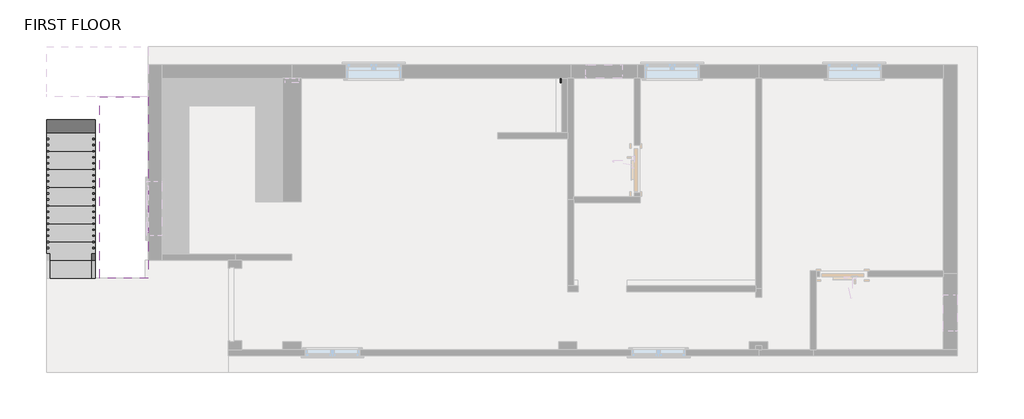
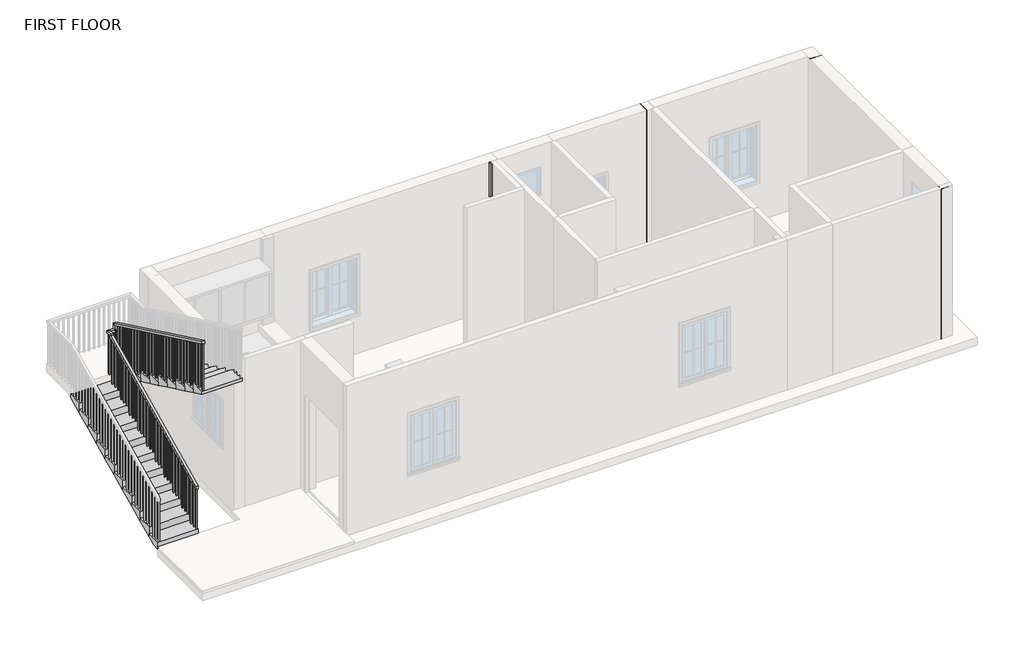
# One storey, part 2 of 3: 4 columns, 2 stair flights, 1 railing.
"""IFC4 building model written with IfcOpenShell, lengths in millimetres."""

from ifc_helpers import new_model, si_unit, frame, origin, place, context, project, spatial, polyline, outline, extrude, faceted_brep, element, save

model = new_model("IFC4")

# Units and contexts
model_context = context("Model", 3, world=origin())
ifc_project = project(units=[si_unit("LENGTHUNIT", "METRE", prefix="MILLI")], contexts=[model_context])

# Site, building, storey
site = spatial("IfcSite", under=ifc_project)
building = spatial("IfcBuilding", under=site)
storey = spatial("IfcBuildingStorey", under=building, Name="FIRST FLOOR", Elevation=3200.4)

# Columns
placement = place(None, origin())
element("IfcColumn", 1, ObjectType="Rectangular Column : 9\" X 12\"", at=placement, inside=storey, context=model_context, shape_type="Brep", body=[
    faceted_brep([(8641.6408773, 5102.5642852, 3200.4), (8870.2408773, 5102.5642852, 3200.4), (8870.2408773, 4797.7642852, 3200.4), (8641.6408773, 4797.7642852, 3200.4), (8641.6408773, 4873.9642852, 3200.4), (8641.6408773, 5102.5642852, 6400.8), (8870.2408773, 5102.5642852, 6400.8), (8870.2408773, 4797.7642852, 6400.8), (8641.6408773, 4797.7642852, 6400.8), (8641.6408773, 4873.9642852, 6400.8)], [[[0, 1, 2, 3, 4]], [[5, 6, 1, 0]], [[6, 7, 2, 1]], [[7, 8, 3, 2]], [[8, 9, 5, 0, 4, 3]], [[5, 9, 8, 7, 6]]]),
])
element("IfcColumn", 2, ObjectType="Rectangular Column : 9\" X 12\"", at=placement, inside=storey, context=model_context, shape_type="Brep", body=[
    faceted_brep([(5390.4408773, 4873.9642852, 3200.4), (5390.4408773, 5102.5642852, 3200.4), (5542.8408773, 5102.5642852, 3200.4), (5542.8408773, 4873.9642852, 3200.4), (5492.0408773, 4873.9642852, 3200.4), (5390.4408773, 4873.9642852, 6400.8), (5390.4408773, 5102.5642852, 6400.8), (5542.8408773, 5102.5642852, 6400.8), (5542.8408773, 4873.9642852, 6400.8), (5492.0408773, 4873.9642852, 6400.8)], [[[0, 1, 2, 3, 4]], [[1, 0, 5, 6]], [[1, 6, 7, 2]], [[5, 0, 4, 3, 8, 9]], [[6, 5, 9, 8, 7]], [[3, 2, 7, 8]]]),
])
element("IfcColumn", 3, ObjectType="Rectangular Column : 9\" X 12\"", at=placement, inside=storey, context=model_context, shape_type="SweptSolid", body=[
    extrude(outline(polyline([(2240.8408773, 4797.7642852), (2215.4408773, 4797.7642852), (2215.4408773, 4873.9642852), (2240.8408773, 4873.9642852), (2240.8408773, 4797.7642852)])), frame((0.0, 0.0, 3200.4), z_axis=(0.0, 0.0, 1.0), x_axis=(1.0, 0.0, 0.0)), (0.0, 0.0, 1.0), 3200.4),
])
element("IfcColumn", 4, ObjectType="Rectangular Column : 9\" X 12\"", at=placement, inside=storey, context=model_context, shape_type="SweptSolid", body=[
    extrude(outline(polyline([(8870.2408773, 225.7642852), (8641.6408773, 225.7642852), (8641.6408773, 327.3642852), (8870.2408773, 327.3642852), (8870.2408773, 225.7642852)])), frame((0.0, 0.0, 3200.4), z_axis=(0.0, 0.0, 1.0), x_axis=(1.0, 0.0, 0.0)), (0.0, 0.0, 1.0), 3200.4),
])

# Railing
element("IfcRailing", 5, ObjectType="Handrail - Rectangular", at=placement, inside=storey, context=model_context, shape_type="SolidModel", body=[
    faceted_brep([(-5633.1591227, 1521.1642852, 4260.2727273), (-5633.1591227, 1521.1642852, 4203.9834559), (-5582.3591227, 1521.1642852, 4203.9834559), (-5582.3591227, 1521.1642852, 4260.2727273), (-5633.1591227, 4492.9642852, 5678.6318182), (-5633.1591227, 4543.7642852, 5646.5880014), (-5582.3591227, 4543.7642852, 5646.5880014), (-5582.3591227, 4492.9642852, 5678.6318182), (-5633.1591227, 4492.9642852, 5715.0), (-5633.1591227, 4543.7642852, 5664.2), (-5582.3591227, 4543.7642852, 5664.2), (-5582.3591227, 4492.9642852, 5715.0), (-5633.1591227, 4619.9642852, 5715.0), (-5633.1591227, 4619.9642852, 5664.2), (-5582.3591227, 4569.1642852, 5664.2), (-5582.3591227, 4569.1642852, 5715.0), (-5506.1591227, 4619.9642852, 5715.0), (-5506.1591227, 4619.9642852, 5664.2), (-5506.1591227, 4569.1642852, 5664.2), (-5506.1591227, 4569.1642852, 5715.0), (-5480.7591227, 4619.9642852, 5715.0), (-5480.7591227, 4569.1642852, 5715.0), (-5480.7591227, 4569.1642852, 5664.2), (-5480.7591227, 4619.9642852, 5664.2)], [[[0, 1, 2, 3]], [[1, 0, 4, 5]], [[2, 1, 5, 6]], [[3, 2, 6, 7]], [[0, 3, 7, 4]], [[5, 4, 8, 9]], [[6, 5, 9, 10]], [[7, 6, 10, 11]], [[4, 7, 11, 8]], [[9, 8, 12, 13]], [[10, 9, 13, 14]], [[11, 10, 14, 15]], [[8, 11, 15, 12]], [[13, 12, 16, 17]], [[14, 13, 17, 18]], [[15, 14, 18, 19]], [[12, 15, 19, 16]], [[20, 21, 22, 23]], [[17, 16, 20, 23]], [[18, 17, 23, 22]], [[19, 18, 22, 21]], [[16, 19, 21, 20]]]),
    faceted_brep([(-5506.1591227, 4619.9642852, 5715.0), (-5455.3591227, 4619.9642852, 5664.2), (-5455.3591227, 4569.1642852, 5664.2), (-5506.1591227, 4569.1642852, 5715.0), (-5506.1591227, 4619.9642852, 5836.2272727), (-5506.1591227, 4569.1642852, 5804.1834559), (-5455.3591227, 4569.1642852, 5804.1834559), (-5455.3591227, 4619.9642852, 5836.2272727)], [[[0, 1, 2, 3]], [[4, 5, 6, 7]], [[1, 0, 4, 7]], [[2, 1, 7, 6]], [[3, 2, 6, 5]], [[0, 3, 5, 4]]]),
    faceted_brep([(-5455.3591227, 4619.9642852, 5836.2272727), (-5455.3591227, 4569.1642852, 5804.1834559), (-5506.1591227, 4569.1642852, 5804.1834559), (-5506.1591227, 4619.9642852, 5836.2272727), (-5455.3591227, 1521.1642852, 7315.2), (-5506.1591227, 1521.1642852, 7315.2), (-5506.1591227, 1521.1642852, 7258.9107287), (-5455.3591227, 1521.1642852, 7258.9107287)], [[[0, 1, 2, 3]], [[4, 5, 6, 7]], [[1, 0, 4, 7]], [[2, 1, 7, 6]], [[3, 2, 6, 5]], [[0, 3, 5, 4]]]),
    extrude(outline(polyline([(1537.0392852, 7251.3340241), (1556.0892852, 7242.2419787), (1556.0892852, 6255.3272727), (1537.0392852, 6255.3272727), (1537.0392852, 7251.3340241)])), frame((-5490.2841227, 0.0, 0.0), z_axis=(1.0, 0.0, 0.0), x_axis=(0.0, 1.0, 0.0)), (0.0, 0.0, 1.0), 19.05),
    extrude(outline(polyline([(1638.6392852, 7202.843115), (1657.6892852, 7193.7510696), (1657.6892852, 6255.3272727), (1638.6392852, 6255.3272727), (1638.6392852, 7202.843115)])), frame((-5490.2841227, 0.0, 0.0), z_axis=(1.0, 0.0, 0.0), x_axis=(0.0, 1.0, 0.0)), (0.0, 0.0, 1.0), 19.05),
    extrude(outline(polyline([(1740.2392852, 7154.3522059), (1759.2892852, 7145.2601605), (1759.2892852, 6255.3272727), (1740.2392852, 6255.3272727), (1740.2392852, 7154.3522059)])), frame((-5490.2841227, 0.0, 0.0), z_axis=(1.0, 0.0, 0.0), x_axis=(0.0, 1.0, 0.0)), (0.0, 0.0, 1.0), 19.05),
    extrude(outline(polyline([(1841.8392852, 7105.8612969), (1860.8892852, 7096.7692514), (1860.8892852, 6109.8545455), (1841.8392852, 6109.8545455), (1841.8392852, 7105.8612969)])), frame((-5490.2841227, 0.0, 0.0), z_axis=(1.0, 0.0, 0.0), x_axis=(0.0, 1.0, 0.0)), (0.0, 0.0, 1.0), 19.05),
    extrude(outline(polyline([(1943.4392852, 7057.3703878), (1962.4892852, 7048.2783423), (1962.4892852, 6109.8545455), (1943.4392852, 6109.8545455), (1943.4392852, 7057.3703878)])), frame((-5490.2841227, 0.0, 0.0), z_axis=(1.0, 0.0, 0.0), x_axis=(0.0, 1.0, 0.0)), (0.0, 0.0, 1.0), 19.05),
    extrude(outline(polyline([(2045.0392852, 7008.8794787), (2064.0892852, 6999.7874332), (2064.0892852, 6109.8545455), (2045.0392852, 6109.8545455), (2045.0392852, 7008.8794787)])), frame((-5490.2841227, 0.0, 0.0), z_axis=(1.0, 0.0, 0.0), x_axis=(0.0, 1.0, 0.0)), (0.0, 0.0, 1.0), 19.05),
    extrude(outline(polyline([(2146.6392852, 6960.3885696), (2165.6892852, 6951.2965241), (2165.6892852, 5964.3818182), (2146.6392852, 5964.3818182), (2146.6392852, 6960.3885696)])), frame((-5490.2841227, 0.0, 0.0), z_axis=(1.0, 0.0, 0.0), x_axis=(0.0, 1.0, 0.0)), (0.0, 0.0, 1.0), 19.05),
    extrude(outline(polyline([(2248.2392852, 6911.8976605), (2267.2892852, 6902.805615), (2267.2892852, 5964.3818182), (2248.2392852, 5964.3818182), (2248.2392852, 6911.8976605)])), frame((-5490.2841227, 0.0, 0.0), z_axis=(1.0, 0.0, 0.0), x_axis=(0.0, 1.0, 0.0)), (0.0, 0.0, 1.0), 19.05),
    extrude(outline(polyline([(2349.8392852, 6863.4067514), (2368.8892852, 6854.3147059), (2368.8892852, 5964.3818182), (2349.8392852, 5964.3818182), (2349.8392852, 6863.4067514)])), frame((-5490.2841227, 0.0, 0.0), z_axis=(1.0, 0.0, 0.0), x_axis=(0.0, 1.0, 0.0)), (0.0, 0.0, 1.0), 19.05),
    extrude(outline(polyline([(2451.4392852, 6814.9158423), (2470.4892852, 6805.8237969), (2470.4892852, 5818.9090909), (2451.4392852, 5818.9090909), (2451.4392852, 6814.9158423)])), frame((-5490.2841227, 0.0, 0.0), z_axis=(1.0, 0.0, 0.0), x_axis=(0.0, 1.0, 0.0)), (0.0, 0.0, 1.0), 19.05),
    extrude(outline(polyline([(2553.0392852, 6766.4249332), (2572.0892852, 6757.3328878), (2572.0892852, 5818.9090909), (2553.0392852, 5818.9090909), (2553.0392852, 6766.4249332)])), frame((-5490.2841227, 0.0, 0.0), z_axis=(1.0, 0.0, 0.0), x_axis=(0.0, 1.0, 0.0)), (0.0, 0.0, 1.0), 19.05),
    extrude(outline(polyline([(2654.6392852, 6717.9340241), (2673.6892852, 6708.8419787), (2673.6892852, 5818.9090909), (2654.6392852, 5818.9090909), (2654.6392852, 6717.9340241)])), frame((-5490.2841227, 0.0, 0.0), z_axis=(1.0, 0.0, 0.0), x_axis=(0.0, 1.0, 0.0)), (0.0, 0.0, 1.0), 19.05),
    extrude(outline(polyline([(2756.2392852, 6669.443115), (2775.2892852, 6660.3510696), (2775.2892852, 5673.4363636), (2756.2392852, 5673.4363636), (2756.2392852, 6669.443115)])), frame((-5490.2841227, 0.0, 0.0), z_axis=(1.0, 0.0, 0.0), x_axis=(0.0, 1.0, 0.0)), (0.0, 0.0, 1.0), 19.05),
    extrude(outline(polyline([(2857.8392852, 6620.9522059), (2876.8892852, 6611.8601605), (2876.8892852, 5673.4363636), (2857.8392852, 5673.4363636), (2857.8392852, 6620.9522059)])), frame((-5490.2841227, 0.0, 0.0), z_axis=(1.0, 0.0, 0.0), x_axis=(0.0, 1.0, 0.0)), (0.0, 0.0, 1.0), 19.05),
    extrude(outline(polyline([(2959.4392852, 6572.4612969), (2978.4892852, 6563.3692514), (2978.4892852, 5673.4363636), (2959.4392852, 5673.4363636), (2959.4392852, 6572.4612969)])), frame((-5490.2841227, 0.0, 0.0), z_axis=(1.0, 0.0, 0.0), x_axis=(0.0, 1.0, 0.0)), (0.0, 0.0, 1.0), 19.05),
    extrude(outline(polyline([(3061.0392852, 6523.9703878), (3080.0892852, 6514.8783423), (3080.0892852, 5527.9636364), (3061.0392852, 5527.9636364), (3061.0392852, 6523.9703878)])), frame((-5490.2841227, 0.0, 0.0), z_axis=(1.0, 0.0, 0.0), x_axis=(0.0, 1.0, 0.0)), (0.0, 0.0, 1.0), 19.05),
    extrude(outline(polyline([(3162.6392852, 6475.4794787), (3181.6892852, 6466.3874332), (3181.6892852, 5527.9636364), (3162.6392852, 5527.9636364), (3162.6392852, 6475.4794787)])), frame((-5490.2841227, 0.0, 0.0), z_axis=(1.0, 0.0, 0.0), x_axis=(0.0, 1.0, 0.0)), (0.0, 0.0, 1.0), 19.05),
    extrude(outline(polyline([(3264.2392852, 6426.9885696), (3283.2892852, 6417.8965241), (3283.2892852, 5527.9636364), (3264.2392852, 5527.9636364), (3264.2392852, 6426.9885696)])), frame((-5490.2841227, 0.0, 0.0), z_axis=(1.0, 0.0, 0.0), x_axis=(0.0, 1.0, 0.0)), (0.0, 0.0, 1.0), 19.05),
    extrude(outline(polyline([(3365.8392852, 6378.4976605), (3384.8892852, 6369.405615), (3384.8892852, 5382.4909091), (3365.8392852, 5382.4909091), (3365.8392852, 6378.4976605)])), frame((-5490.2841227, 0.0, 0.0), z_axis=(1.0, 0.0, 0.0), x_axis=(0.0, 1.0, 0.0)), (0.0, 0.0, 1.0), 19.05),
    extrude(outline(polyline([(3467.4392852, 6330.0067514), (3486.4892852, 6320.9147059), (3486.4892852, 5382.4909091), (3467.4392852, 5382.4909091), (3467.4392852, 6330.0067514)])), frame((-5490.2841227, 0.0, 0.0), z_axis=(1.0, 0.0, 0.0), x_axis=(0.0, 1.0, 0.0)), (0.0, 0.0, 1.0), 19.05),
    extrude(outline(polyline([(3569.0392852, 6281.5158423), (3588.0892852, 6272.4237969), (3588.0892852, 5382.4909091), (3569.0392852, 5382.4909091), (3569.0392852, 6281.5158423)])), frame((-5490.2841227, 0.0, 0.0), z_axis=(1.0, 0.0, 0.0), x_axis=(0.0, 1.0, 0.0)), (0.0, 0.0, 1.0), 19.05),
    extrude(outline(polyline([(3670.6392852, 6233.0249332), (3689.6892852, 6223.9328878), (3689.6892852, 5237.0181818), (3670.6392852, 5237.0181818), (3670.6392852, 6233.0249332)])), frame((-5490.2841227, 0.0, 0.0), z_axis=(1.0, 0.0, 0.0), x_axis=(0.0, 1.0, 0.0)), (0.0, 0.0, 1.0), 19.05),
    extrude(outline(polyline([(3772.2392852, 6184.5340241), (3791.2892852, 6175.4419787), (3791.2892852, 5237.0181818), (3772.2392852, 5237.0181818), (3772.2392852, 6184.5340241)])), frame((-5490.2841227, 0.0, 0.0), z_axis=(1.0, 0.0, 0.0), x_axis=(0.0, 1.0, 0.0)), (0.0, 0.0, 1.0), 19.05),
    extrude(outline(polyline([(3873.8392852, 6136.043115), (3892.8892852, 6126.9510696), (3892.8892852, 5237.0181818), (3873.8392852, 5237.0181818), (3873.8392852, 6136.043115)])), frame((-5490.2841227, 0.0, 0.0), z_axis=(1.0, 0.0, 0.0), x_axis=(0.0, 1.0, 0.0)), (0.0, 0.0, 1.0), 19.05),
    extrude(outline(polyline([(3975.4392852, 6087.5522059), (3994.4892852, 6078.4601605), (3994.4892852, 5091.5454545), (3975.4392852, 5091.5454545), (3975.4392852, 6087.5522059)])), frame((-5490.2841227, 0.0, 0.0), z_axis=(1.0, 0.0, 0.0), x_axis=(0.0, 1.0, 0.0)), (0.0, 0.0, 1.0), 19.05),
    extrude(outline(polyline([(4077.0392852, 6039.0612969), (4096.0892852, 6029.9692514), (4096.0892852, 5091.5454545), (4077.0392852, 5091.5454545), (4077.0392852, 6039.0612969)])), frame((-5490.2841227, 0.0, 0.0), z_axis=(1.0, 0.0, 0.0), x_axis=(0.0, 1.0, 0.0)), (0.0, 0.0, 1.0), 19.05),
    extrude(outline(polyline([(4178.6392852, 5990.5703878), (4197.6892852, 5981.4783423), (4197.6892852, 5091.5454545), (4178.6392852, 5091.5454545), (4178.6392852, 5990.5703878)])), frame((-5490.2841227, 0.0, 0.0), z_axis=(1.0, 0.0, 0.0), x_axis=(0.0, 1.0, 0.0)), (0.0, 0.0, 1.0), 19.05),
    extrude(outline(polyline([(4280.2392852, 5942.0794787), (4299.2892852, 5932.9874332), (4299.2892852, 4946.0727273), (4280.2392852, 4946.0727273), (4280.2392852, 5942.0794787)])), frame((-5490.2841227, 0.0, 0.0), z_axis=(1.0, 0.0, 0.0), x_axis=(0.0, 1.0, 0.0)), (0.0, 0.0, 1.0), 19.05),
    extrude(outline(polyline([(4381.8392852, 5893.5885696), (4400.8892852, 5884.4965241), (4400.8892852, 4946.0727273), (4381.8392852, 4946.0727273), (4381.8392852, 5893.5885696)])), frame((-5490.2841227, 0.0, 0.0), z_axis=(1.0, 0.0, 0.0), x_axis=(0.0, 1.0, 0.0)), (0.0, 0.0, 1.0), 19.05),
    extrude(outline(polyline([(4483.4392852, 5845.0976605), (4502.4892852, 5836.005615), (4502.4892852, 4946.0727273), (4483.4392852, 4946.0727273), (4483.4392852, 5845.0976605)])), frame((-5490.2841227, 0.0, 0.0), z_axis=(1.0, 0.0, 0.0), x_axis=(0.0, 1.0, 0.0)), (0.0, 0.0, 1.0), 19.05),
    extrude(outline(polyline([(-5515.6841227, 4585.0392852), (-5515.6841227, 4604.0892852), (-5496.6341227, 4604.0892852), (-5496.6341227, 4585.0392852), (-5515.6841227, 4585.0392852)])), frame((0.0, 0.0, 4800.6), z_axis=(0.0, 0.0, 1.0), x_axis=(1.0, 0.0, 0.0)), (0.0, 0.0, 1.0), 863.6),
    extrude(outline(polyline([(-5598.2341227, 4559.6392852), (-5617.2841227, 4559.6392852), (-5617.2841227, 4578.6892852), (-5598.2341227, 4578.6892852), (-5598.2341227, 4559.6392852)])), frame((0.0, 0.0, 4800.6), z_axis=(0.0, 0.0, 1.0), x_axis=(1.0, 0.0, 0.0)), (0.0, 0.0, 1.0), 863.6),
    extrude(outline(polyline([(4458.0392852, 5605.6737969), (4477.0892852, 5614.7658423), (4477.0892852, 4655.1272727), (4458.0392852, 4655.1272727), (4458.0392852, 5605.6737969)])), frame((-5617.2841227, 0.0, 0.0), z_axis=(1.0, 0.0, 0.0), x_axis=(0.0, 1.0, 0.0)), (0.0, 0.0, 1.0), 19.05),
    extrude(outline(polyline([(4356.4392852, 5557.1828878), (4375.4892852, 5566.2749332), (4375.4892852, 4655.1272727), (4356.4392852, 4655.1272727), (4356.4392852, 5557.1828878)])), frame((-5617.2841227, 0.0, 0.0), z_axis=(1.0, 0.0, 0.0), x_axis=(0.0, 1.0, 0.0)), (0.0, 0.0, 1.0), 19.05),
    extrude(outline(polyline([(4254.8392852, 5508.6919787), (4273.8892852, 5517.7840241), (4273.8892852, 4655.1272727), (4254.8392852, 4655.1272727), (4254.8392852, 5508.6919787)])), frame((-5617.2841227, 0.0, 0.0), z_axis=(1.0, 0.0, 0.0), x_axis=(0.0, 1.0, 0.0)), (0.0, 0.0, 1.0), 19.05),
    extrude(outline(polyline([(4153.2392852, 5460.2010696), (4172.2892852, 5469.293115), (4172.2892852, 4509.6545455), (4153.2392852, 4509.6545455), (4153.2392852, 5460.2010696)])), frame((-5617.2841227, 0.0, 0.0), z_axis=(1.0, 0.0, 0.0), x_axis=(0.0, 1.0, 0.0)), (0.0, 0.0, 1.0), 19.05),
    extrude(outline(polyline([(4051.6392852, 5411.7101605), (4070.6892852, 5420.8022059), (4070.6892852, 4509.6545455), (4051.6392852, 4509.6545455), (4051.6392852, 5411.7101605)])), frame((-5617.2841227, 0.0, 0.0), z_axis=(1.0, 0.0, 0.0), x_axis=(0.0, 1.0, 0.0)), (0.0, 0.0, 1.0), 19.05),
    extrude(outline(polyline([(3950.0392852, 5363.2192514), (3969.0892852, 5372.3112969), (3969.0892852, 4509.6545455), (3950.0392852, 4509.6545455), (3950.0392852, 5363.2192514)])), frame((-5617.2841227, 0.0, 0.0), z_axis=(1.0, 0.0, 0.0), x_axis=(0.0, 1.0, 0.0)), (0.0, 0.0, 1.0), 19.05),
    extrude(outline(polyline([(3848.4392852, 5314.7283423), (3867.4892852, 5323.8203878), (3867.4892852, 4364.1818182), (3848.4392852, 4364.1818182), (3848.4392852, 5314.7283423)])), frame((-5617.2841227, 0.0, 0.0), z_axis=(1.0, 0.0, 0.0), x_axis=(0.0, 1.0, 0.0)), (0.0, 0.0, 1.0), 19.05),
    extrude(outline(polyline([(3746.8392852, 5266.2374332), (3765.8892852, 5275.3294787), (3765.8892852, 4364.1818182), (3746.8392852, 4364.1818182), (3746.8392852, 5266.2374332)])), frame((-5617.2841227, 0.0, 0.0), z_axis=(1.0, 0.0, 0.0), x_axis=(0.0, 1.0, 0.0)), (0.0, 0.0, 1.0), 19.05),
    extrude(outline(polyline([(3645.2392852, 5217.7465241), (3664.2892852, 5226.8385696), (3664.2892852, 4364.1818182), (3645.2392852, 4364.1818182), (3645.2392852, 5217.7465241)])), frame((-5617.2841227, 0.0, 0.0), z_axis=(1.0, 0.0, 0.0), x_axis=(0.0, 1.0, 0.0)), (0.0, 0.0, 1.0), 19.05),
    extrude(outline(polyline([(3543.6392852, 5169.255615), (3562.6892852, 5178.3476605), (3562.6892852, 4218.7090909), (3543.6392852, 4218.7090909), (3543.6392852, 5169.255615)])), frame((-5617.2841227, 0.0, 0.0), z_axis=(1.0, 0.0, 0.0), x_axis=(0.0, 1.0, 0.0)), (0.0, 0.0, 1.0), 19.05),
    extrude(outline(polyline([(3442.0392852, 5120.7647059), (3461.0892852, 5129.8567514), (3461.0892852, 4218.7090909), (3442.0392852, 4218.7090909), (3442.0392852, 5120.7647059)])), frame((-5617.2841227, 0.0, 0.0), z_axis=(1.0, 0.0, 0.0), x_axis=(0.0, 1.0, 0.0)), (0.0, 0.0, 1.0), 19.05),
    extrude(outline(polyline([(3340.4392852, 5072.2737969), (3359.4892852, 5081.3658423), (3359.4892852, 4218.7090909), (3340.4392852, 4218.7090909), (3340.4392852, 5072.2737969)])), frame((-5617.2841227, 0.0, 0.0), z_axis=(1.0, 0.0, 0.0), x_axis=(0.0, 1.0, 0.0)), (0.0, 0.0, 1.0), 19.05),
    extrude(outline(polyline([(3238.8392852, 5023.7828878), (3257.8892852, 5032.8749332), (3257.8892852, 4073.2363636), (3238.8392852, 4073.2363636), (3238.8392852, 5023.7828878)])), frame((-5617.2841227, 0.0, 0.0), z_axis=(1.0, 0.0, 0.0), x_axis=(0.0, 1.0, 0.0)), (0.0, 0.0, 1.0), 19.05),
    extrude(outline(polyline([(3137.2392852, 4975.2919787), (3156.2892852, 4984.3840241), (3156.2892852, 4073.2363636), (3137.2392852, 4073.2363636), (3137.2392852, 4975.2919787)])), frame((-5617.2841227, 0.0, 0.0), z_axis=(1.0, 0.0, 0.0), x_axis=(0.0, 1.0, 0.0)), (0.0, 0.0, 1.0), 19.05),
    extrude(outline(polyline([(3035.6392852, 4926.8010696), (3054.6892852, 4935.893115), (3054.6892852, 4073.2363636), (3035.6392852, 4073.2363636), (3035.6392852, 4926.8010696)])), frame((-5617.2841227, 0.0, 0.0), z_axis=(1.0, 0.0, 0.0), x_axis=(0.0, 1.0, 0.0)), (0.0, 0.0, 1.0), 19.05),
    extrude(outline(polyline([(2934.0392852, 4878.3101605), (2953.0892852, 4887.4022059), (2953.0892852, 3927.7636364), (2934.0392852, 3927.7636364), (2934.0392852, 4878.3101605)])), frame((-5617.2841227, 0.0, 0.0), z_axis=(1.0, 0.0, 0.0), x_axis=(0.0, 1.0, 0.0)), (0.0, 0.0, 1.0), 19.05),
    extrude(outline(polyline([(2832.4392852, 4829.8192514), (2851.4892852, 4838.9112969), (2851.4892852, 3927.7636364), (2832.4392852, 3927.7636364), (2832.4392852, 4829.8192514)])), frame((-5617.2841227, 0.0, 0.0), z_axis=(1.0, 0.0, 0.0), x_axis=(0.0, 1.0, 0.0)), (0.0, 0.0, 1.0), 19.05),
    extrude(outline(polyline([(2730.8392852, 4781.3283423), (2749.8892852, 4790.4203878), (2749.8892852, 3927.7636364), (2730.8392852, 3927.7636364), (2730.8392852, 4781.3283423)])), frame((-5617.2841227, 0.0, 0.0), z_axis=(1.0, 0.0, 0.0), x_axis=(0.0, 1.0, 0.0)), (0.0, 0.0, 1.0), 19.05),
    extrude(outline(polyline([(2629.2392852, 4732.8374332), (2648.2892852, 4741.9294787), (2648.2892852, 3782.2909091), (2629.2392852, 3782.2909091), (2629.2392852, 4732.8374332)])), frame((-5617.2841227, 0.0, 0.0), z_axis=(1.0, 0.0, 0.0), x_axis=(0.0, 1.0, 0.0)), (0.0, 0.0, 1.0), 19.05),
    extrude(outline(polyline([(2527.6392852, 4684.3465241), (2546.6892852, 4693.4385696), (2546.6892852, 3782.2909091), (2527.6392852, 3782.2909091), (2527.6392852, 4684.3465241)])), frame((-5617.2841227, 0.0, 0.0), z_axis=(1.0, 0.0, 0.0), x_axis=(0.0, 1.0, 0.0)), (0.0, 0.0, 1.0), 19.05),
    extrude(outline(polyline([(2426.0392852, 4635.855615), (2445.0892852, 4644.9476605), (2445.0892852, 3782.2909091), (2426.0392852, 3782.2909091), (2426.0392852, 4635.855615)])), frame((-5617.2841227, 0.0, 0.0), z_axis=(1.0, 0.0, 0.0), x_axis=(0.0, 1.0, 0.0)), (0.0, 0.0, 1.0), 19.05),
    extrude(outline(polyline([(2324.4392852, 4587.3647059), (2343.4892852, 4596.4567514), (2343.4892852, 3636.8181818), (2324.4392852, 3636.8181818), (2324.4392852, 4587.3647059)])), frame((-5617.2841227, 0.0, 0.0), z_axis=(1.0, 0.0, 0.0), x_axis=(0.0, 1.0, 0.0)), (0.0, 0.0, 1.0), 19.05),
    extrude(outline(polyline([(2222.8392852, 4538.8737969), (2241.8892852, 4547.9658423), (2241.8892852, 3636.8181818), (2222.8392852, 3636.8181818), (2222.8392852, 4538.8737969)])), frame((-5617.2841227, 0.0, 0.0), z_axis=(1.0, 0.0, 0.0), x_axis=(0.0, 1.0, 0.0)), (0.0, 0.0, 1.0), 19.05),
    extrude(outline(polyline([(2121.2392852, 4490.3828878), (2140.2892852, 4499.4749332), (2140.2892852, 3636.8181818), (2121.2392852, 3636.8181818), (2121.2392852, 4490.3828878)])), frame((-5617.2841227, 0.0, 0.0), z_axis=(1.0, 0.0, 0.0), x_axis=(0.0, 1.0, 0.0)), (0.0, 0.0, 1.0), 19.05),
    extrude(outline(polyline([(2019.6392852, 4441.8919787), (2038.6892852, 4450.9840241), (2038.6892852, 3491.3454545), (2019.6392852, 3491.3454545), (2019.6392852, 4441.8919787)])), frame((-5617.2841227, 0.0, 0.0), z_axis=(1.0, 0.0, 0.0), x_axis=(0.0, 1.0, 0.0)), (0.0, 0.0, 1.0), 19.05),
    extrude(outline(polyline([(1918.0392852, 4393.4010696), (1937.0892852, 4402.493115), (1937.0892852, 3491.3454545), (1918.0392852, 3491.3454545), (1918.0392852, 4393.4010696)])), frame((-5617.2841227, 0.0, 0.0), z_axis=(1.0, 0.0, 0.0), x_axis=(0.0, 1.0, 0.0)), (0.0, 0.0, 1.0), 19.05),
    extrude(outline(polyline([(1816.4392852, 4344.9101605), (1835.4892852, 4354.0022059), (1835.4892852, 3491.3454545), (1816.4392852, 3491.3454545), (1816.4392852, 4344.9101605)])), frame((-5617.2841227, 0.0, 0.0), z_axis=(1.0, 0.0, 0.0), x_axis=(0.0, 1.0, 0.0)), (0.0, 0.0, 1.0), 19.05),
    extrude(outline(polyline([(1714.8392852, 4296.4192514), (1733.8892852, 4305.5112969), (1733.8892852, 3345.8727273), (1714.8392852, 3345.8727273), (1714.8392852, 4296.4192514)])), frame((-5617.2841227, 0.0, 0.0), z_axis=(1.0, 0.0, 0.0), x_axis=(0.0, 1.0, 0.0)), (0.0, 0.0, 1.0), 19.05),
    extrude(outline(polyline([(1613.2392852, 4247.9283423), (1632.2892852, 4257.0203878), (1632.2892852, 3345.8727273), (1613.2392852, 3345.8727273), (1613.2392852, 4247.9283423)])), frame((-5617.2841227, 0.0, 0.0), z_axis=(1.0, 0.0, 0.0), x_axis=(0.0, 1.0, 0.0)), (0.0, 0.0, 1.0), 19.05),
    extrude(outline(polyline([(-5490.2841227, 4585.0392852), (-5490.2841227, 4604.0892852), (-5471.2341227, 4604.0892852), (-5471.2341227, 4585.0392852), (-5490.2841227, 4585.0392852)])), frame((0.0, 0.0, 4800.6), z_axis=(0.0, 0.0, 1.0), x_axis=(1.0, 0.0, 0.0)), (0.0, 0.0, 1.0), 863.6),
    extrude(outline(polyline([(-5598.2341227, 4585.0392852), (-5617.2841227, 4585.0392852), (-5617.2841227, 4604.0892852), (-5598.2341227, 4604.0892852), (-5598.2341227, 4585.0392852)])), frame((0.0, 0.0, 4800.6), z_axis=(0.0, 0.0, 1.0), x_axis=(1.0, 0.0, 0.0)), (0.0, 0.0, 1.0), 863.6),
    extrude(outline(polyline([(1521.1642852, 7258.9107287), (1540.2142852, 7249.8186832), (1540.2142852, 6255.3272727), (1521.1642852, 6255.3272727), (1521.1642852, 7258.9107287)])), frame((-5490.2841227, 0.0, 0.0), z_axis=(1.0, 0.0, 0.0), x_axis=(0.0, 1.0, 0.0)), (0.0, 0.0, 1.0), 19.05),
    extrude(outline(polyline([(1521.1642852, 4203.9834559), (1540.2142852, 4213.0755014), (1540.2142852, 3345.8727273), (1521.1642852, 3345.8727273), (1521.1642852, 4203.9834559)])), frame((-5617.2841227, 0.0, 0.0), z_axis=(1.0, 0.0, 0.0), x_axis=(0.0, 1.0, 0.0)), (0.0, 0.0, 1.0), 19.05),
])

# Stair flights
element("IfcStairFlight", 6, ObjectType="3/4\" Nosing", at=placement, inside=storey, context=model_context, shape_type="Brep", body=[
    faceted_brep([(-6395.1591227, 1825.9642852, 3345.8727273), (-6395.1591227, 1521.1642852, 3345.8727273), (-5582.3591227, 1521.1642852, 3345.8727273), (-5582.3591227, 1825.9642852, 3345.8727273), (-6395.1591227, 1825.9642852, 3275.5111381), (-6395.1591227, 1668.5885672, 3200.4), (-6395.1591227, 1521.1642852, 3200.4), (-5582.3591227, 1521.1642852, 3200.4), (-5582.3591227, 1668.5885672, 3200.4), (-5582.3591227, 1825.9642852, 3275.5111381), (-6395.1591227, 2130.7642852, 3491.3454545), (-6395.1591227, 1825.9642852, 3491.3454545), (-5582.3591227, 1825.9642852, 3491.3454545), (-5582.3591227, 2130.7642852, 3491.3454545), (-6395.1591227, 2130.7642852, 3420.9838654), (-5582.3591227, 2130.7642852, 3420.9838654), (-6395.1591227, 2435.5642852, 3636.8181818), (-6395.1591227, 2130.7642852, 3636.8181818), (-5582.3591227, 2130.7642852, 3636.8181818), (-5582.3591227, 2435.5642852, 3636.8181818), (-6395.1591227, 2435.5642852, 3566.4565927), (-5582.3591227, 2435.5642852, 3566.4565927), (-6395.1591227, 2740.3642852, 3782.2909091), (-6395.1591227, 2435.5642852, 3782.2909091), (-5582.3591227, 2435.5642852, 3782.2909091), (-5582.3591227, 2740.3642852, 3782.2909091), (-6395.1591227, 2740.3642852, 3711.9293199), (-5582.3591227, 2740.3642852, 3711.9293199), (-6395.1591227, 3045.1642852, 3927.7636364), (-6395.1591227, 2740.3642852, 3927.7636364), (-5582.3591227, 2740.3642852, 3927.7636364), (-5582.3591227, 3045.1642852, 3927.7636364), (-6395.1591227, 3045.1642852, 3857.4020472), (-5582.3591227, 3045.1642852, 3857.4020472), (-6395.1591227, 3349.9642852, 4073.2363636), (-6395.1591227, 3045.1642852, 4073.2363636), (-5582.3591227, 3045.1642852, 4073.2363636), (-5582.3591227, 3349.9642852, 4073.2363636), (-6395.1591227, 3349.9642852, 4002.8747745), (-5582.3591227, 3349.9642852, 4002.8747745), (-6395.1591227, 3654.7642852, 4218.7090909), (-6395.1591227, 3349.9642852, 4218.7090909), (-5582.3591227, 3349.9642852, 4218.7090909), (-5582.3591227, 3654.7642852, 4218.7090909), (-6395.1591227, 3654.7642852, 4148.3475018), (-5582.3591227, 3654.7642852, 4148.3475018), (-6395.1591227, 3959.5642852, 4364.1818182), (-6395.1591227, 3654.7642852, 4364.1818182), (-5582.3591227, 3654.7642852, 4364.1818182), (-5582.3591227, 3959.5642852, 4364.1818182), (-6395.1591227, 3959.5642852, 4293.820229), (-5582.3591227, 3959.5642852, 4293.820229), (-6395.1591227, 4264.3642852, 4439.2929563), (-6395.1591227, 4569.1642852, 4584.7656836), (-5582.3591227, 4569.1642852, 4584.7656836), (-5582.3591227, 4264.3642852, 4439.2929563), (-6395.1591227, 4264.3642852, 4509.6545455), (-6395.1591227, 3959.5642852, 4509.6545455), (-5582.3591227, 3959.5642852, 4509.6545455), (-5582.3591227, 4264.3642852, 4509.6545455), (-6395.1591227, 4569.1642852, 4655.1272727), (-6395.1591227, 4264.3642852, 4655.1272727), (-5582.3591227, 4264.3642852, 4655.1272727), (-5582.3591227, 4569.1642852, 4655.1272727), (-5582.3591227, 4569.1642852, 4622.8)], [[[0, 1, 2, 3]], [[1, 0, 4, 5, 6]], [[2, 1, 6, 7]], [[3, 2, 7, 8, 9]], [[10, 11, 12, 13]], [[11, 10, 14, 4, 0]], [[0, 3, 12, 11]], [[13, 12, 3, 9, 15]], [[16, 17, 18, 19]], [[17, 16, 20, 14, 10]], [[10, 13, 18, 17]], [[19, 18, 13, 15, 21]], [[22, 23, 24, 25]], [[23, 22, 26, 20, 16]], [[16, 19, 24, 23]], [[25, 24, 19, 21, 27]], [[28, 29, 30, 31]], [[29, 28, 32, 26, 22]], [[22, 25, 30, 29]], [[31, 30, 25, 27, 33]], [[34, 35, 36, 37]], [[35, 34, 38, 32, 28]], [[28, 31, 36, 35]], [[37, 36, 31, 33, 39]], [[40, 41, 42, 43]], [[41, 40, 44, 38, 34]], [[34, 37, 42, 41]], [[43, 42, 37, 39, 45]], [[46, 47, 48, 49]], [[47, 46, 50, 44, 40]], [[40, 43, 48, 47]], [[49, 48, 43, 45, 51]], [[7, 6, 5, 8]], [[8, 5, 4, 14, 20, 26, 32, 38, 44, 50, 52, 53, 54, 55, 51, 45, 39, 33, 27, 21, 15, 9]], [[56, 57, 58, 59]], [[57, 56, 52, 50, 46]], [[46, 49, 58, 57]], [[59, 58, 49, 51, 55]], [[60, 61, 62, 63]], [[61, 60, 53, 52, 56]], [[56, 59, 62, 61]], [[63, 62, 59, 55, 54, 64]], [[60, 63, 64, 54, 53]]]),
])
element("IfcStairFlight", 7, ObjectType="3/4\" Nosing", at=placement, inside=storey, context=model_context, shape_type="Brep", body=[
    faceted_brep([(-4693.3591227, 4264.3642852, 4946.0727273), (-4693.3591227, 4569.1642852, 4946.0727273), (-5506.1591227, 4569.1642852, 4946.0727273), (-5506.1591227, 4264.3642852, 4946.0727273), (-4693.3591227, 4264.3642852, 4875.7111381), (-4693.3591227, 4569.1642852, 4730.2384108), (-4693.3591227, 4569.1642852, 4800.6), (-5506.1591227, 4569.1642852, 4730.2384108), (-5506.1591227, 4264.3642852, 4875.7111381), (-4693.3591227, 3959.5642852, 5091.5454545), (-4693.3591227, 4264.3642852, 5091.5454545), (-5506.1591227, 4264.3642852, 5091.5454545), (-5506.1591227, 3959.5642852, 5091.5454545), (-4693.3591227, 3959.5642852, 5021.1838654), (-5506.1591227, 3959.5642852, 5021.1838654), (-4693.3591227, 3654.7642852, 5237.0181818), (-4693.3591227, 3959.5642852, 5237.0181818), (-5506.1591227, 3959.5642852, 5237.0181818), (-5506.1591227, 3654.7642852, 5237.0181818), (-4693.3591227, 3654.7642852, 5166.6565927), (-5506.1591227, 3654.7642852, 5166.6565927), (-4693.3591227, 3349.9642852, 5382.4909091), (-4693.3591227, 3654.7642852, 5382.4909091), (-5506.1591227, 3654.7642852, 5382.4909091), (-5506.1591227, 3349.9642852, 5382.4909091), (-4693.3591227, 3349.9642852, 5312.1293199), (-5506.1591227, 3349.9642852, 5312.1293199), (-4693.3591227, 3045.1642852, 5527.9636364), (-4693.3591227, 3349.9642852, 5527.9636364), (-5506.1591227, 3349.9642852, 5527.9636364), (-5506.1591227, 3045.1642852, 5527.9636364), (-4693.3591227, 3045.1642852, 5457.6020472), (-5506.1591227, 3045.1642852, 5457.6020472), (-4693.3591227, 2740.3642852, 5673.4363636), (-4693.3591227, 3045.1642852, 5673.4363636), (-5506.1591227, 3045.1642852, 5673.4363636), (-5506.1591227, 2740.3642852, 5673.4363636), (-4693.3591227, 2740.3642852, 5603.0747745), (-5506.1591227, 2740.3642852, 5603.0747745), (-4693.3591227, 2435.5642852, 5818.9090909), (-4693.3591227, 2740.3642852, 5818.9090909), (-5506.1591227, 2740.3642852, 5818.9090909), (-5506.1591227, 2435.5642852, 5818.9090909), (-4693.3591227, 2435.5642852, 5748.5475018), (-5506.1591227, 2435.5642852, 5748.5475018), (-4693.3591227, 2130.7642852, 5964.3818182), (-4693.3591227, 2435.5642852, 5964.3818182), (-5506.1591227, 2435.5642852, 5964.3818182), (-5506.1591227, 2130.7642852, 5964.3818182), (-4693.3591227, 2130.7642852, 5894.020229), (-5506.1591227, 2130.7642852, 5894.020229), (-4693.3591227, 1825.9642852, 6039.4929563), (-4693.3591227, 1521.1642852, 6184.9656836), (-5506.1591227, 1521.1642852, 6184.9656836), (-5506.1591227, 1825.9642852, 6039.4929563), (-4693.3591227, 1825.9642852, 6109.8545455), (-4693.3591227, 2130.7642852, 6109.8545455), (-5506.1591227, 2130.7642852, 6109.8545455), (-5506.1591227, 1825.9642852, 6109.8545455), (-4693.3591227, 1521.1642852, 6255.3272727), (-4693.3591227, 1825.9642852, 6255.3272727), (-5506.1591227, 1825.9642852, 6255.3272727), (-5506.1591227, 1521.1642852, 6255.3272727)], [[[0, 1, 2, 3]], [[1, 0, 4, 5, 6]], [[2, 1, 6, 5, 7]], [[3, 2, 7, 8]], [[9, 10, 11, 12]], [[10, 9, 13, 4, 0]], [[11, 10, 0, 3]], [[12, 11, 3, 8, 14]], [[15, 16, 17, 18]], [[16, 15, 19, 13, 9]], [[17, 16, 9, 12]], [[18, 17, 12, 14, 20]], [[21, 22, 23, 24]], [[22, 21, 25, 19, 15]], [[23, 22, 15, 18]], [[24, 23, 18, 20, 26]], [[27, 28, 29, 30]], [[28, 27, 31, 25, 21]], [[29, 28, 21, 24]], [[30, 29, 24, 26, 32]], [[33, 34, 35, 36]], [[34, 33, 37, 31, 27]], [[35, 34, 27, 30]], [[36, 35, 30, 32, 38]], [[39, 40, 41, 42]], [[40, 39, 43, 37, 33]], [[41, 40, 33, 36]], [[42, 41, 36, 38, 44]], [[45, 46, 47, 48]], [[46, 45, 49, 43, 39]], [[47, 46, 39, 42]], [[48, 47, 42, 44, 50]], [[5, 4, 13, 19, 25, 31, 37, 43, 49, 51, 52, 53, 54, 50, 44, 38, 32, 26, 20, 14, 8, 7]], [[55, 56, 57, 58]], [[56, 55, 51, 49, 45]], [[57, 56, 45, 48]], [[58, 57, 48, 50, 54]], [[59, 60, 61, 62]], [[60, 59, 52, 51, 55]], [[61, 60, 55, 58]], [[62, 61, 58, 54, 53]], [[59, 62, 53, 52]]]),
])

save(model, "model.ifc")

# Revit data of these elements
# Type "Rectangular Column : 9\" X 12\""
#   Assembly Code = "B1010200"
#   Depth = 0' - 9"
#   Offset Base = 0' - 0"
#   Offset Top = 0' - 0"
#   Width = 1' - 0"
#   Material = none
# Type "Handrail - Rectangular"
#   Assembly Code = "C2010400"
#   built-in parameter 1008612 = 0.0416667 (stored number, unit not read)
#   built-in parameter 1008611 = 0.0416667 (stored number, unit not read)
#   built-in parameter 1008609 = 0.333333 (stored number, unit not read)
#   built-in parameter 1008604 = 0.166667 (stored number, unit not read)
#   built-in parameter 1008603 = 0.166667 (stored number, unit not read)
#   Railing Height = 3' - 0"
#   built-in parameter 1008630 = 2
#   built-in parameter 1008610 = 2
#   built-in parameter 1008618 = Baluster - Square : 3/4"
# Elements 1, 2, 4 (IfcColumn, "Rectangular Column : 9\" X 12\"")
#   Phase Created = New Construction
#   Materials on its faces: "Brick, Common"
# Element 3 (IfcColumn, "Rectangular Column : 9\" X 12\"")
#   Phase Created = New Construction
#   Materials on its faces: "Brick, Common", "lite white"
# Element 5 (IfcRailing, "Handrail - Rectangular")
#   Phase Created = New Construction
# Elements 6, 7 (IfcStairFlight, "3/4\" Nosing")
#   Phase Created = New Construction
#   Materials on its faces: "Concrete, Cast-in-Place gray"
# Materials
#   "Brick, Common": class "Masonry", colour RGB 170 98 104, transparency 0, Description = "Common brick", Cost = 0
#   "lite white": class "Generic", colour RGB 120 120 120, transparency 0, Cost = 0
#   "Concrete, Cast-in-Place gray": class "Concrete", colour RGB 192 192 192, transparency 0, Description = "Cast-in-place concrete", Cost = 0
